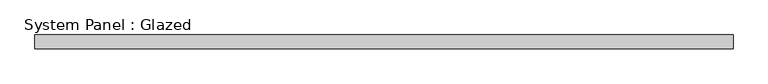
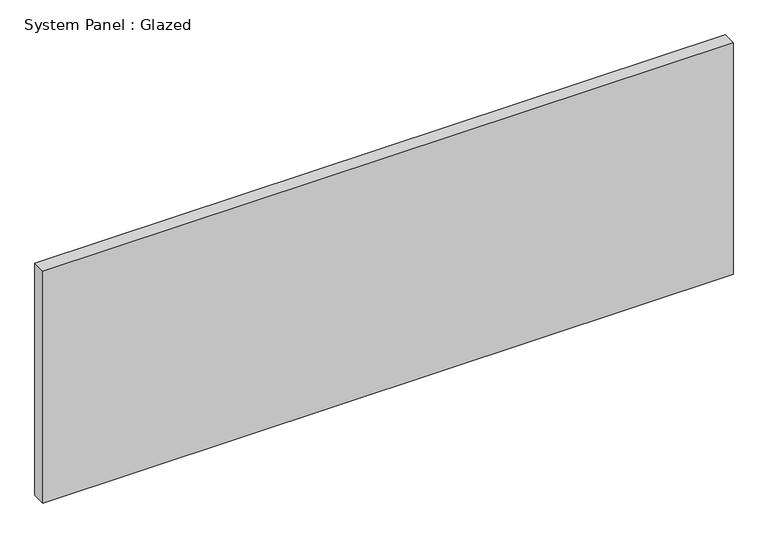
"""IFC4 building model written with IfcOpenShell, lengths in millimetres: plate geometry, System Panel : Glazed."""

from ifc_helpers import new_model, si_unit, origin, origin_with_axes, place, context, project, spatial, polyline, outline, extrude, source, transform, mapped, element, save


def system_panel_glazed_ac301e25(model_context):
    return source(origin(), model_context, "Body", "SweptSolid", [
        extrude(outline(polyline([(638.1750001, 19.05), (-638.1750001, 19.05), (-638.1750001, 44.45), (638.1750001, 44.45), (638.1750001, 19.05)])), origin_with_axes(), (0.0, 0.0, 1.0), 452.9666667),
    ])


if __name__ == "__main__":
    model = new_model("IFC4")
    model_context = context("Model", 3, world=origin())
    ifc_project = project(units=[si_unit("LENGTHUNIT", "METRE", prefix="MILLI")], contexts=[model_context])
    site = spatial("IfcSite", under=ifc_project)
    building = spatial("IfcBuilding", under=site)
    placement = place(None, origin())
    system_panel_glazed_shape = system_panel_glazed_ac301e25(model_context)
    element("IfcPlate", 1, ObjectType="System Panel : Glazed", at=placement, inside=building, context=model_context, shape_type="MappedRepresentation", body=[
        mapped(system_panel_glazed_shape, transform((0.0, 0.0, 0.0), x_axis=(1.0, 0.0, 0.0), y_axis=(0.0, 1.0, 0.0), z_axis=(0.0, 0.0, 1.0))),
    ])
    save(model, "model.ifc")

# Revit data of these elements
# Type "System Panel : Glazed"
#   Construction Type Id = "GSP4R"
#   Analytic Construction = "1/8 in Pilkington single glazing"
#   Visual Light Transmittance = 0.9
#   Solar Heat Gain Coefficient = 0.86
#   Heat Transfer Coefficient (U) = 1.18115 BTU/(h·ft²·°F)
#   Define Thermal Properties by = 1
# Element 1 (IfcPlate, "System Panel : Glazed")
#   Materials on its faces: "glass panel 223"
# Materials
#   "glass panel 223": class "Generic", colour RGB 120 120 120, transparency 0, Cost = 0
